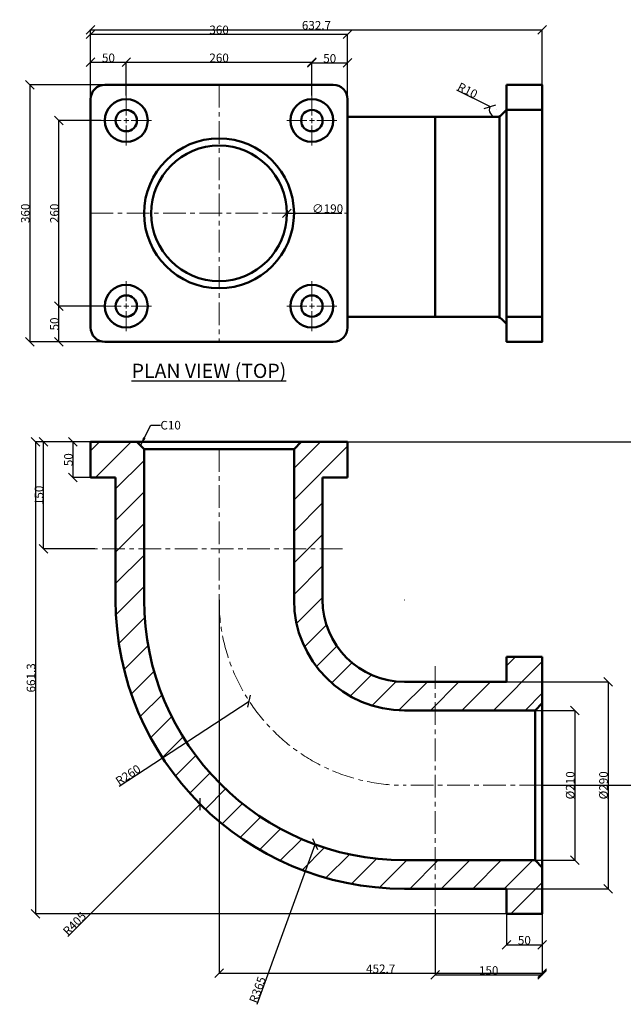
# Model space of a CAD drawing. Units: millimetres. Extents: x 509 to 2033, y 349 to 1731.
# Tile 1 of 2: x 509 to 1355, y 352 to 1731. Entities that reach past the tile are written whole.
import ezdxf

# ---------------------------------------------------------------- set-up
doc = ezdxf.new("R2010")
doc.units = ezdxf.units.MM
doc.header["$MEASUREMENT"] = 0
doc.linetypes.add('CENTER', pattern=[50.8, 31.75, -6.35, 6.35, -6.35])
for name, color, linetype, lineweight in [('M-CNTR', 1, 'CENTER', 18), ('M-DIMS', 2, 'Continuous', 25), ('M-HATC', 8, 'Continuous', 18), ('M-OUTL', 7, 'Continuous', 50), ('M-TEXT', 7, 'Continuous', 25)]:
    doc.layers.add(name, color=color, linetype=linetype, lineweight=lineweight)
doc.styles.get("Standard").update_dxf_attribs({"font": 'arial.ttf'})
doc.dimstyles.get("Standard").update_dxf_attribs({"dimtxt": 12, "dimasz": 12, "dimexe": 0.18, "dimexo": 0.0625, "dimgap": 0.09, "dimtad": 1, "dimdec": 0, "dimzin": 0, "dimdsep": 46, "dimtxsty": 'Standard', "dimblk": 'OBLIQUE', "dimcen": 0.09, "dimclre": 251, "dimadec": 0, "dimazin": 0, "dimtfac": 1, "dimtdec": 0, "dimtofl": 0, "dimtmove": 0, "dimatfit": 3, "dimfxl": 1, "dimtolj": 1, "dimtzin": 0, "dimarcsym": 0})

# ---------------------------------------------------------------- blocks, each defined once
blk = doc.blocks.new('*U2')
at = {"layer": 'M-CNTR', "color": 0, "transparency": 16777216}
for p, q in [((0, 7), (0, 35.12)), ((-35.12, 0), (-7, 0)), ((7, 0), (35.12, 0)), ((0, -35.12), (0, -7))]:
    blk.add_line(p, q, dxfattribs=at)
at = {"layer": 'M-CNTR', "color": 0, "linetype": 'Continuous', "transparency": 16777216}
for p, q in [((-3.5, 0), (3.5, 0)), ((0, -3.5), (0, 3.5))]:
    blk.add_line(p, q, dxfattribs=at)
blk = doc.blocks.new('*U3')
at = {"layer": 'M-CNTR', "color": 0, "transparency": 16777216}
for p, q in [((0, 7), (0, 35.12)), ((-35.12, 0), (-7, 0)), ((7, 0), (35.12, 0)), ((0, -35.12), (0, -7))]:
    blk.add_line(p, q, dxfattribs=at)
at = {"layer": 'M-CNTR', "color": 0, "linetype": 'Continuous', "transparency": 16777216}
for p, q in [((-3.5, 0), (3.5, 0)), ((0, -3.5), (0, 3.5))]:
    blk.add_line(p, q, dxfattribs=at)
blk = doc.blocks.new('*U4')
at = {"layer": 'M-CNTR', "color": 0, "transparency": 16777216}
for p, q in [((0, 7), (0, 35.12)), ((-35.12, 0), (-7, 0)), ((7, 0), (35.12, 0)), ((0, -35.12), (0, -7))]:
    blk.add_line(p, q, dxfattribs=at)
at = {"layer": 'M-CNTR', "color": 0, "linetype": 'Continuous', "transparency": 16777216}
for p, q in [((-3.5, 0), (3.5, 0)), ((0, -3.5), (0, 3.5))]:
    blk.add_line(p, q, dxfattribs=at)
blk = doc.blocks.new('*U5')
at = {"layer": 'M-CNTR', "color": 0, "transparency": 16777216}
for p, q in [((0, 7), (0, 35.12)), ((-35.12, 0), (-7, 0)), ((7, 0), (35.12, 0)), ((0, -35.12), (0, -7))]:
    blk.add_line(p, q, dxfattribs=at)
at = {"layer": 'M-CNTR', "color": 0, "linetype": 'Continuous', "transparency": 16777216}
for p, q in [((-3.5, 0), (3.5, 0)), ((0, -3.5), (0, 3.5))]:
    blk.add_line(p, q, dxfattribs=at)
blk = doc.blocks.new('_Oblique')
at = {"color": 0, "linetype": 'ByBlock', "lineweight": -2}
blk.add_line((-0.5, -0.5), (0.5, 0.5), dxfattribs=at)
blk = doc.blocks.new('*D10')
at = {"layer": 'Defpoints', "color": 0, "transparency": 16777216}
for p in [(563.7, 1590.1), (623.1, 1590.1), (623.1, 1330.1)]:
    blk.add_point(p, dxfattribs=at)
at = {"layer": 'M-DIMS', "color": 0, "lineweight": -2, "transparency": 16777216}
for p, q in [((623, 1590.1), (563.5, 1590.1)), ((563.7, 1330.1), (563.7, 1590.1)), ((623, 1330.1), (563.5, 1330.1))]:
    blk.add_line(p, q, dxfattribs=at)
at = {"layer": 'M-DIMS', "color": 0, "lineweight": -2, "transparency": 16777216, "xscale": 12, "yscale": 12, "zscale": 12}
for p, rotation in [((563.7, 1590.1), 90), ((563.7, 1330.1), 270)]:
    blk.add_blockref('_Oblique', p, dxfattribs=dict(at, rotation=rotation))
at = {"layer": 'M-DIMS', "color": 0, "transparency": 16777216, "insert": (557.5, 1460.1), "char_height": 12, "attachment_point": 5, "rotation": 90}
blk.add_mtext('\\A1;260', dxfattribs=at)
blk = doc.blocks.new('*D11')
at = {"layer": 'Defpoints', "color": 0, "transparency": 16777216}
for p in [(563.7, 1330.1), (628.2, 1330.1), (628.2, 1280.1)]:
    blk.add_point(p, dxfattribs=at)
at = {"layer": 'M-DIMS', "color": 0, "lineweight": -2, "transparency": 16777216}
for p, q in [((628.1, 1330.1), (563.5, 1330.1)), ((563.7, 1280.1), (563.7, 1330.1)), ((628.1, 1280.1), (563.5, 1280.1))]:
    blk.add_line(p, q, dxfattribs=at)
at = {"layer": 'M-DIMS', "color": 0, "lineweight": -2, "transparency": 16777216, "xscale": 12, "yscale": 12, "zscale": 12}
for p, rotation in [((563.7, 1330.1), 90), ((563.7, 1280.1), 270)]:
    blk.add_blockref('_Oblique', p, dxfattribs=dict(at, rotation=rotation))
at = {"layer": 'M-DIMS', "color": 0, "transparency": 16777216, "insert": (557.5, 1305.1), "char_height": 12, "attachment_point": 5, "rotation": 90}
blk.add_mtext('\\A1;50', dxfattribs=at)
blk = doc.blocks.new('*D12')
at = {"layer": 'Defpoints', "color": 0, "transparency": 16777216}
for p in [(628.2, 1640.1), (522.9, 1280.1), (639, 1280.1)]:
    blk.add_point(p, dxfattribs=at)
at = {"layer": 'M-DIMS', "color": 0, "lineweight": -2, "transparency": 16777216}
for p, q in [((628.1, 1640.1), (522.8, 1640.1)), ((522.9, 1640.1), (522.9, 1280.1)), ((639, 1280.1), (522.8, 1280.1))]:
    blk.add_line(p, q, dxfattribs=at)
at = {"layer": 'M-DIMS', "color": 0, "lineweight": -2, "transparency": 16777216, "xscale": 12, "yscale": 12, "zscale": 12}
for p, rotation in [((522.9, 1640.1), 90), ((522.9, 1280.1), 270)]:
    blk.add_blockref('_Oblique', p, dxfattribs=dict(at, rotation=rotation))
at = {"layer": 'M-DIMS', "color": 0, "transparency": 16777216, "insert": (516.7, 1460.1), "char_height": 12, "attachment_point": 5, "rotation": 90}
blk.add_mtext('\\A1;360', dxfattribs=at)
blk = doc.blocks.new('*D13')
at = {"layer": 'Defpoints', "color": 0, "transparency": 16777216}
for p in [(968.2, 1711), (608.2, 1620.1), (968.2, 1620.1)]:
    blk.add_point(p, dxfattribs=at)
at = {"layer": 'M-DIMS', "color": 0, "lineweight": -2, "transparency": 16777216}
for p, q in [((608.2, 1620.2), (608.2, 1711.2)), ((608.2, 1711), (968.2, 1711)), ((968.2, 1620.2), (968.2, 1711.2))]:
    blk.add_line(p, q, dxfattribs=at)
at = {"layer": 'M-DIMS', "color": 0, "lineweight": -2, "transparency": 16777216, "xscale": 12, "yscale": 12, "zscale": 12, "rotation": 180}
blk.add_blockref('_Oblique', (608.2, 1711), dxfattribs=at)
at = {"layer": 'M-DIMS', "color": 0, "lineweight": -2, "transparency": 16777216, "xscale": 12, "yscale": 12, "zscale": 12}
blk.add_blockref('_Oblique', (968.2, 1711), dxfattribs=at)
at = {"layer": 'M-DIMS', "color": 0, "transparency": 16777216, "insert": (788.2, 1717.2), "char_height": 12, "attachment_point": 5}
blk.add_mtext('\\A1;360', dxfattribs=at)
blk = doc.blocks.new('*D14')
at = {"layer": 'Defpoints', "color": 0, "transparency": 16777216}
for p in [(658.2, 1671.8), (608.2, 1620.1), (658.2, 1625.2)]:
    blk.add_point(p, dxfattribs=at)
at = {"layer": 'M-DIMS', "color": 0, "lineweight": -2, "transparency": 16777216}
for p, q in [((608.2, 1620.2), (608.2, 1672)), ((608.2, 1671.8), (658.2, 1671.8)), ((658.2, 1625.3), (658.2, 1672))]:
    blk.add_line(p, q, dxfattribs=at)
at = {"layer": 'M-DIMS', "color": 0, "lineweight": -2, "transparency": 16777216, "xscale": 12, "yscale": 12, "zscale": 12, "rotation": 180}
blk.add_blockref('_Oblique', (608.2, 1671.8), dxfattribs=at)
at = {"layer": 'M-DIMS', "color": 0, "lineweight": -2, "transparency": 16777216, "xscale": 12, "yscale": 12, "zscale": 12}
blk.add_blockref('_Oblique', (658.2, 1671.8), dxfattribs=at)
at = {"layer": 'M-DIMS', "color": 0, "transparency": 16777216, "insert": (633.2, 1678), "char_height": 12, "attachment_point": 5}
blk.add_mtext('\\A1;50', dxfattribs=at)
blk = doc.blocks.new('*D15')
at = {"layer": 'Defpoints', "color": 0, "transparency": 16777216}
for p in [(658.2, 1671.8), (918.2, 1671.8), (918.2, 1625.2)]:
    blk.add_point(p, dxfattribs=at)
at = {"layer": 'M-DIMS', "color": 0, "lineweight": -2, "transparency": 16777216}
for p, q in [((658.2, 1671.9), (658.2, 1672)), ((658.2, 1671.8), (918.2, 1671.8)), ((918.2, 1625.3), (918.2, 1672))]:
    blk.add_line(p, q, dxfattribs=at)
at = {"layer": 'M-DIMS', "color": 0, "lineweight": -2, "transparency": 16777216, "xscale": 12, "yscale": 12, "zscale": 12, "rotation": 180}
blk.add_blockref('_Oblique', (658.2, 1671.8), dxfattribs=at)
at = {"layer": 'M-DIMS', "color": 0, "lineweight": -2, "transparency": 16777216, "xscale": 12, "yscale": 12, "zscale": 12}
blk.add_blockref('_Oblique', (918.2, 1671.8), dxfattribs=at)
at = {"layer": 'M-DIMS', "color": 0, "transparency": 16777216, "insert": (788.2, 1678), "char_height": 12, "attachment_point": 5}
blk.add_mtext('\\A1;260', dxfattribs=at)
blk = doc.blocks.new('*D16')
at = {"layer": 'Defpoints', "color": 0, "transparency": 16777216}
for p in [(968.2, 1671), (918.2, 1625.2), (968.2, 1620.1)]:
    blk.add_point(p, dxfattribs=at)
at = {"layer": 'M-DIMS', "color": 0, "lineweight": -2, "transparency": 16777216}
for p, q in [((918.2, 1625.3), (918.2, 1671.1)), ((918.2, 1671), (968.2, 1671)), ((968.2, 1620.2), (968.2, 1671.1))]:
    blk.add_line(p, q, dxfattribs=at)
at = {"layer": 'M-DIMS', "color": 0, "lineweight": -2, "transparency": 16777216, "xscale": 12, "yscale": 12, "zscale": 12, "rotation": 180}
blk.add_blockref('_Oblique', (918.2, 1671), dxfattribs=at)
at = {"layer": 'M-DIMS', "color": 0, "lineweight": -2, "transparency": 16777216, "xscale": 12, "yscale": 12, "zscale": 12}
blk.add_blockref('_Oblique', (968.2, 1671), dxfattribs=at)
at = {"layer": 'M-DIMS', "color": 0, "transparency": 16777216, "insert": (943.2, 1677.2), "char_height": 12, "attachment_point": 5}
blk.add_mtext('\\A1;50', dxfattribs=at)
blk = doc.blocks.new('*D17')
at = {"layer": 'Defpoints', "color": 0, "transparency": 16777216}
for p in [(1167.8, 1609.6), (1176.8, 1605.1)]:
    blk.add_point(p, dxfattribs=at)
at = {"layer": 'M-DIMS', "color": 0, "lineweight": -2, "transparency": 16777216}
for p, q in [((1120.6, 1633.2), (1167.8, 1609.6)), ((1176.7, 1605.1), (1176.9, 1605.1)), ((1176.8, 1605), (1176.8, 1605.2))]:
    blk.add_line(p, q, dxfattribs=at)
blk.add_arc((1176.8, 1605.1), 10, 152.4068, 269.6419, dxfattribs=at)
at = {"layer": 'M-DIMS', "color": 0, "lineweight": -2, "transparency": 16777216, "xscale": 12, "yscale": 12, "zscale": 12, "rotation": 333.4380769186279}
blk.add_blockref('_Oblique', (1167.8, 1609.6), dxfattribs=at)
at = {"layer": 'M-DIMS', "color": 0, "transparency": 16777216, "insert": (1136.3, 1632.3), "char_height": 12, "attachment_point": 5, "rotation": 333.4381}
blk.add_mtext('\\A1;R10', dxfattribs=at)
blk = doc.blocks.new('*D18')
at = {"layer": 'Defpoints', "color": 0, "transparency": 16777216}
for p in [(542.1, 1139.9), (608.2, 1139.9), (614.3, 989.9)]:
    blk.add_point(p, dxfattribs=at)
at = {"layer": 'M-DIMS', "color": 0, "lineweight": -2, "transparency": 16777216}
for p, q in [((608.1, 1139.9), (541.9, 1139.9)), ((542.1, 989.9), (542.1, 1139.9)), ((614.2, 989.9), (541.9, 989.9))]:
    blk.add_line(p, q, dxfattribs=at)
at = {"layer": 'M-DIMS', "color": 0, "lineweight": -2, "transparency": 16777216, "xscale": 12, "yscale": 12, "zscale": 12}
for p, rotation in [((542.1, 1139.9), 90), ((542.1, 989.9), 270)]:
    blk.add_blockref('_Oblique', p, dxfattribs=dict(at, rotation=rotation))
at = {"layer": 'M-DIMS', "color": 0, "transparency": 16777216, "insert": (535.9, 1064.9), "char_height": 12, "attachment_point": 5, "rotation": 90}
blk.add_mtext('\\A1;150', dxfattribs=at)
blk = doc.blocks.new('*D19')
at = {"layer": 'Defpoints', "color": 0, "transparency": 16777216}
for p in [(608.2, 1139.9), (583.3, 1089.9), (608.2, 1089.9)]:
    blk.add_point(p, dxfattribs=at)
at = {"layer": 'M-DIMS', "color": 0, "lineweight": -2, "transparency": 16777216}
for p, q in [((608.1, 1139.9), (583.1, 1139.9)), ((583.3, 1139.9), (583.3, 1089.9)), ((608.1, 1089.9), (583.1, 1089.9))]:
    blk.add_line(p, q, dxfattribs=at)
at = {"layer": 'M-DIMS', "color": 0, "lineweight": -2, "transparency": 16777216, "xscale": 12, "yscale": 12, "zscale": 12}
for p, rotation in [((583.3, 1139.9), 90), ((583.3, 1089.9), 270)]:
    blk.add_blockref('_Oblique', p, dxfattribs=dict(at, rotation=rotation))
at = {"layer": 'M-DIMS', "color": 0, "transparency": 16777216, "insert": (577.1, 1114.9), "char_height": 12, "attachment_point": 5, "rotation": 90}
blk.add_mtext('\\A1;50', dxfattribs=at)
blk = doc.blocks.new('*D20')
at = {"layer": 'Defpoints', "color": 0, "transparency": 16777216}
for p in [(1048.2, 918.6), (830.4, 776.5)]:
    blk.add_point(p, dxfattribs=at)
at = {"layer": 'M-DIMS', "color": 0, "lineweight": -2, "transparency": 16777216}
for p, q in [((1048.1, 918.6), (1048.3, 918.6)), ((1048.2, 918.5), (1048.2, 918.7)), ((648.1, 657.6), (830.4, 776.5))]:
    blk.add_line(p, q, dxfattribs=at)
at = {"layer": 'M-DIMS', "color": 0, "lineweight": -2, "transparency": 16777216, "xscale": 12, "yscale": 12, "zscale": 12, "rotation": 33.11996082454108}
blk.add_blockref('_Oblique', (830.4, 776.5), dxfattribs=at)
at = {"layer": 'M-DIMS', "color": 0, "transparency": 16777216, "insert": (660.7, 673.2), "char_height": 12, "attachment_point": 5, "rotation": 33.12}
blk.add_mtext('\\A1;R260', dxfattribs=at)
blk = doc.blocks.new('*D21')
at = {"layer": 'Defpoints', "color": 0, "transparency": 16777216}
for p in [(1190.9, 478.6), (1240.9, 478.6), (1240.9, 435.2)]:
    blk.add_point(p, dxfattribs=at)
at = {"layer": 'M-DIMS', "color": 0, "lineweight": -2, "transparency": 16777216}
for p, q in [((1190.9, 478.5), (1190.9, 435)), ((1240.9, 478.5), (1240.9, 435)), ((1190.9, 435.2), (1240.9, 435.2))]:
    blk.add_line(p, q, dxfattribs=at)
at = {"layer": 'M-DIMS', "color": 0, "lineweight": -2, "transparency": 16777216, "xscale": 12, "yscale": 12, "zscale": 12, "rotation": 180}
blk.add_blockref('_Oblique', (1190.9, 435.2), dxfattribs=at)
at = {"layer": 'M-DIMS', "color": 0, "lineweight": -2, "transparency": 16777216, "xscale": 12, "yscale": 12, "zscale": 12}
blk.add_blockref('_Oblique', (1240.9, 435.2), dxfattribs=at)
at = {"layer": 'M-DIMS', "color": 0, "transparency": 16777216, "insert": (1215.9, 441.4), "char_height": 12, "attachment_point": 5}
blk.add_mtext('\\A1;50', dxfattribs=at)
blk = doc.blocks.new('*D22')
at = {"layer": 'Defpoints', "color": 0, "transparency": 16777216}
for p in [(1090.9, 484.9), (1240.9, 478.6), (1240.9, 392.9)]:
    blk.add_point(p, dxfattribs=at)
at = {"layer": 'M-DIMS', "color": 0, "lineweight": -2, "transparency": 16777216}
for p, q in [((1090.9, 484.9), (1090.9, 392.7)), ((1240.9, 478.5), (1240.9, 392.7)), ((1090.9, 392.9), (1240.9, 392.9))]:
    blk.add_line(p, q, dxfattribs=at)
at = {"layer": 'M-DIMS', "color": 0, "lineweight": -2, "transparency": 16777216, "xscale": 12, "yscale": 12, "zscale": 12, "rotation": 180}
blk.add_blockref('_Oblique', (1090.9, 392.9), dxfattribs=at)
at = {"layer": 'M-DIMS', "color": 0, "lineweight": -2, "transparency": 16777216, "xscale": 12, "yscale": 12, "zscale": 12}
blk.add_blockref('_Oblique', (1240.9, 392.9), dxfattribs=at)
at = {"layer": 'M-DIMS', "color": 0, "transparency": 16777216, "insert": (1165.9, 399.1), "char_height": 12, "attachment_point": 5}
blk.add_mtext('\\A1;150', dxfattribs=at)
blk = doc.blocks.new('*D23')
at = {"layer": 'Defpoints', "color": 0, "transparency": 16777216}
for p in [(1230.9, 763.6), (1230.9, 553.6), (1286.6, 553.6)]:
    blk.add_point(p, dxfattribs=at)
at = {"layer": 'M-DIMS', "color": 0, "lineweight": -2, "transparency": 16777216}
for p, q in [((1231, 763.6), (1286.8, 763.6)), ((1286.6, 763.6), (1286.6, 553.6)), ((1231, 553.6), (1286.8, 553.6))]:
    blk.add_line(p, q, dxfattribs=at)
at = {"layer": 'M-DIMS', "color": 0, "lineweight": -2, "transparency": 16777216, "xscale": 12, "yscale": 12, "zscale": 12}
for p, rotation in [((1286.6, 763.6), 90), ((1286.6, 553.6), 270)]:
    blk.add_blockref('_Oblique', p, dxfattribs=dict(at, rotation=rotation))
at = {"layer": 'M-DIMS', "color": 0, "transparency": 16777216, "insert": (1280.1, 658.6), "char_height": 12, "attachment_point": 5, "rotation": 90}
blk.add_mtext('\\A1;%%C210', dxfattribs=at)
blk = doc.blocks.new('*D24')
at = {"layer": 'Defpoints', "color": 0, "transparency": 16777216}
for p in [(1190.9, 803.6), (1190.9, 513.6), (1333.3, 513.6)]:
    blk.add_point(p, dxfattribs=at)
at = {"layer": 'M-DIMS', "color": 0, "lineweight": -2, "transparency": 16777216}
for p, q in [((1191, 803.6), (1333.5, 803.6)), ((1333.3, 803.6), (1333.3, 513.6)), ((1191, 513.6), (1333.5, 513.6))]:
    blk.add_line(p, q, dxfattribs=at)
at = {"layer": 'M-DIMS', "color": 0, "lineweight": -2, "transparency": 16777216, "xscale": 12, "yscale": 12, "zscale": 12}
for p, rotation in [((1333.3, 803.6), 90), ((1333.3, 513.6), 270)]:
    blk.add_blockref('_Oblique', p, dxfattribs=dict(at, rotation=rotation))
at = {"layer": 'M-DIMS', "color": 0, "transparency": 16777216, "insert": (1326.7, 658.6), "char_height": 12, "attachment_point": 5, "rotation": 90}
blk.add_mtext('\\A1;%%C290', dxfattribs=at)
blk = doc.blocks.new('BOLT-HOLE-CBORE')
for radius in [30, 15]:
    blk.add_circle((30, 30), radius)
blk = doc.blocks.new('*D35')
at = {"layer": 'Defpoints', "color": 0, "transparency": 16777216}
for p in [(968.2, 1139.9), (1240.9, 658.6), (1981, 658.6)]:
    blk.add_point(p, dxfattribs=at)
at = {"layer": 'M-DIMS', "color": 251, "lineweight": -2, "transparency": 16777216}
for p, q in [((968.2, 1139.9), (1981.1, 1139.9)), ((1241, 658.6), (1981.1, 658.6))]:
    blk.add_line(p, q, dxfattribs=at)
at = {"layer": 'M-DIMS', "color": 0, "lineweight": -2, "transparency": 16777216}
blk.add_line((1981, 1139.9), (1981, 658.6), dxfattribs=at)
at = {"layer": 'M-DIMS', "color": 0, "lineweight": -2, "transparency": 16777216, "xscale": 12, "yscale": 12, "zscale": 12}
for p, rotation in [((1981, 1139.9), 90), ((1981, 658.6), 270)]:
    blk.add_blockref('_Oblique', p, dxfattribs=dict(at, rotation=rotation))
at = {"layer": 'M-DIMS', "color": 0, "transparency": 16777216, "insert": (1974.7, 899.2), "char_height": 12, "attachment_point": 5, "rotation": 90}
blk.add_mtext('\\A1;481.3', dxfattribs=at)
blk = doc.blocks.new('*D36')
at = {"layer": 'Defpoints', "color": 0, "transparency": 16777216}
for p in [(788.2, 918.6), (1240.9, 478.6), (1240.9, 395.3)]:
    blk.add_point(p, dxfattribs=at)
at = {"layer": 'M-DIMS', "color": 251, "lineweight": -2, "transparency": 16777216}
for p, q in [((788.2, 918.5), (788.2, 395.1)), ((1240.9, 478.5), (1240.9, 395.1))]:
    blk.add_line(p, q, dxfattribs=at)
at = {"layer": 'M-DIMS', "color": 0, "lineweight": -2, "transparency": 16777216}
blk.add_line((788.2, 395.3), (1240.9, 395.3), dxfattribs=at)
at = {"layer": 'M-DIMS', "color": 0, "lineweight": -2, "transparency": 16777216, "xscale": 12, "yscale": 12, "zscale": 12, "rotation": 180}
blk.add_blockref('_Oblique', (788.2, 395.3), dxfattribs=at)
at = {"layer": 'M-DIMS', "color": 0, "lineweight": -2, "transparency": 16777216, "xscale": 12, "yscale": 12, "zscale": 12}
blk.add_blockref('_Oblique', (1240.9, 395.3), dxfattribs=at)
at = {"layer": 'M-DIMS', "color": 0, "transparency": 16777216, "insert": (1014.6, 401.5), "char_height": 12, "attachment_point": 5}
blk.add_mtext('\\A1;452.7', dxfattribs=at)
blk = doc.blocks.new('*D37')
at = {"layer": 'Defpoints', "color": 0, "transparency": 16777216}
for p in [(608.2, 1139.9), (530.9, 478.6), (1240.9, 478.6)]:
    blk.add_point(p, dxfattribs=at)
at = {"layer": 'M-DIMS', "color": 251, "lineweight": -2, "transparency": 16777216}
for p, q in [((608.1, 1139.9), (530.8, 1139.9)), ((1240.9, 478.6), (530.8, 478.6))]:
    blk.add_line(p, q, dxfattribs=at)
at = {"layer": 'M-DIMS', "color": 0, "lineweight": -2, "transparency": 16777216}
blk.add_line((530.9, 1139.9), (530.9, 478.6), dxfattribs=at)
at = {"layer": 'M-DIMS', "color": 0, "lineweight": -2, "transparency": 16777216, "xscale": 12, "yscale": 12, "zscale": 12}
for p, rotation in [((530.9, 1139.9), 90), ((530.9, 478.6), 270)]:
    blk.add_blockref('_Oblique', p, dxfattribs=dict(at, rotation=rotation))
at = {"layer": 'M-DIMS', "color": 0, "transparency": 16777216, "insert": (524.7, 809.2), "char_height": 12, "attachment_point": 5, "rotation": 90}
blk.add_mtext('\\A1;661.3', dxfattribs=at)
blk = doc.blocks.new('*D38')
at = {"layer": 'Defpoints', "color": 0, "transparency": 16777216}
for p in [(1240.9, 1717.4), (1240.9, 1640.1), (608.2, 1620.1)]:
    blk.add_point(p, dxfattribs=at)
at = {"layer": 'M-DIMS', "color": 251, "lineweight": -2, "transparency": 16777216}
for p, q in [((608.2, 1620.2), (608.2, 1717.6)), ((1240.9, 1640.2), (1240.9, 1717.6))]:
    blk.add_line(p, q, dxfattribs=at)
at = {"layer": 'M-DIMS', "color": 0, "lineweight": -2, "transparency": 16777216}
blk.add_line((608.2, 1717.4), (1240.9, 1717.4), dxfattribs=at)
at = {"layer": 'M-DIMS', "color": 0, "lineweight": -2, "transparency": 16777216, "xscale": 12, "yscale": 12, "zscale": 12, "rotation": 180}
blk.add_blockref('_Oblique', (608.2, 1717.4), dxfattribs=at)
at = {"layer": 'M-DIMS', "color": 0, "lineweight": -2, "transparency": 16777216, "xscale": 12, "yscale": 12, "zscale": 12}
blk.add_blockref('_Oblique', (1240.9, 1717.4), dxfattribs=at)
at = {"layer": 'M-DIMS', "color": 0, "transparency": 16777216, "insert": (924.6, 1723.6), "char_height": 12, "attachment_point": 5}
blk.add_mtext('\\A1;632.7', dxfattribs=at)
blk = doc.blocks.new('*D39')
at = {"layer": 'Defpoints', "color": 0, "transparency": 16777216}
for p in [(1048.2, 918.6), (761.8, 632.2)]:
    blk.add_point(p, dxfattribs=at)
at = {"layer": 'M-DIMS', "color": 251, "lineweight": -2, "transparency": 16777216}
for p, q in [((1048.1, 918.6), (1048.3, 918.6)), ((1048.2, 918.5), (1048.2, 918.7))]:
    blk.add_line(p, q, dxfattribs=at)
at = {"layer": 'M-DIMS', "color": 0, "lineweight": -2, "transparency": 16777216}
blk.add_line((576.4, 446.9), (761.8, 632.2), dxfattribs=at)
at = {"layer": 'M-DIMS', "color": 0, "lineweight": -2, "transparency": 16777216, "xscale": 12, "yscale": 12, "zscale": 12, "rotation": 44.99999749912137}
blk.add_blockref('_Oblique', (761.8, 632.2), dxfattribs=at)
at = {"layer": 'M-DIMS', "color": 0, "transparency": 16777216, "insert": (585.6, 464.8), "char_height": 12, "attachment_point": 5, "rotation": 45}
blk.add_mtext('\\A1;R405', dxfattribs=at)
blk = doc.blocks.new('*D40')
at = {"layer": 'Defpoints', "color": 0, "transparency": 16777216}
for p in [(1048.2, 918.6), (923, 575.7)]:
    blk.add_point(p, dxfattribs=at)
at = {"layer": 'M-DIMS', "color": 251, "lineweight": -2, "transparency": 16777216}
for p, q in [((1048.1, 918.6), (1048.3, 918.6)), ((1048.2, 918.5), (1048.2, 918.7))]:
    blk.add_line(p, q, dxfattribs=at)
at = {"layer": 'M-DIMS', "color": 0, "lineweight": -2, "transparency": 16777216}
blk.add_line((841.4, 352), (923, 575.7), dxfattribs=at)
at = {"layer": 'M-DIMS', "color": 0, "lineweight": -2, "transparency": 16777216, "xscale": 12, "yscale": 12, "zscale": 12, "rotation": 69.95038313699236}
blk.add_blockref('_Oblique', (923, 575.7), dxfattribs=at)
at = {"layer": 'M-DIMS', "color": 0, "transparency": 16777216, "insert": (842.1, 372.1), "char_height": 12, "attachment_point": 5, "rotation": 69.9504}
blk.add_mtext('\\A1;R365', dxfattribs=at)
blk = doc.blocks.new('*D41')
at = {"layer": 'Defpoints', "color": 0, "transparency": 16777216}
for p in [(693.2, 1460.1), (883.2, 1460.1)]:
    blk.add_point(p, dxfattribs=at)
at = {"layer": 'M-DIMS', "color": 251, "lineweight": -2, "transparency": 16777216}
for p, q in [((788.1, 1460.1), (788.3, 1460.1)), ((788.2, 1460), (788.2, 1460.2))]:
    blk.add_line(p, q, dxfattribs=at)
at = {"layer": 'M-DIMS', "color": 0, "lineweight": -2, "transparency": 16777216}
blk.add_line((960, 1460.1), (883.2, 1460.1), dxfattribs=at)
at = {"layer": 'M-DIMS', "color": 0, "lineweight": -2, "transparency": 16777216, "xscale": 12, "yscale": 12, "zscale": 12, "rotation": 180.0001025292896}
blk.add_blockref('_Oblique', (883.2, 1460.1), dxfattribs=at)
at = {"layer": 'M-DIMS', "color": 0, "transparency": 16777216, "insert": (940.2, 1466.7), "char_height": 12, "attachment_point": 5, "rotation": 0.0001}
blk.add_mtext('\\A1;∅190', dxfattribs=at)

msp = doc.modelspace()

# ---------------------------------------------------------------- hatches: boundary and pattern name
at = {"layer": 'M-HATC'}
h = msp.add_hatch(dxfattribs=at)
h.set_pattern_fill('ANSI31', color=256, scale=250)
h.set_pattern_definition([(45, (92.202, 1053.204), (-22.0971, 22.0971), [])])
h.paths.add_polyline_path([(683.18, 1129.86), (673.18, 1139.86), (608.18, 1139.86), (608.18, 1089.86), (643.18, 1089.86), (643.18, 989.86), (683.18, 989.86)])
h.paths.add_polyline_path([(933.18, 1089.86), (968.18, 1089.86), (968.18, 1139.86), (903.18, 1139.86), (893.18, 1129.86), (893.18, 989.86), (933.18, 989.86)])
h.paths.add_polyline_path([(933.18, 918.61), (933.18, 989.86), (893.18, 989.86), (893.18, 918.61, 0.4142136), (1048.18, 763.61), (1230.92, 763.61), (1240.92, 773.61), (1240.92, 838.61), (1190.92, 838.61), (1190.92, 803.61), (1048.18, 803.61, -0.4142136)])
h.paths.add_polyline_path([(1240.92, 543.61), (1230.92, 553.61), (1048.18, 553.61, -0.4142136), (683.18, 918.61), (683.18, 989.86), (643.18, 989.86), (643.18, 918.61, 0.4142136), (1048.18, 513.61), (1190.92, 513.61), (1190.92, 478.61), (1240.92, 478.61)])

# ---------------------------------------------------------------- linework, layer by layer
at = {"layer": 'M-CNTR'}
for p, q in [((788.18, 1640.13), (788.18, 1280.13)), ((608.18, 1460.13), (968.18, 1460.13)), ((788.18, 1129.86), (788.18, 918.61)), ((960.98, 989.86), (614.3, 989.86)), ((1090.92, 825.75), (1090.92, 484.93)), ((1240.92, 658.61), (1048.18, 658.61))]:
    msp.add_line(p, q, dxfattribs=at)
msp.add_arc((1048.18, 918.61), 260, 180, 270, dxfattribs=at)
at = {"layer": 'M-OUTL'}
for p, q in [((1190.92, 1605.13), (1183.85, 1598.06)), ((1190.92, 1605.13), (1240.92, 1605.13)), ((1176.78, 1595.13), (968.18, 1595.13)), ((1090.92, 1315.13), (1090.92, 1595.13)), ((1180.92, 1314.23), (1180.92, 1596.03)), ((1176.78, 1315.13), (968.18, 1315.13)), ((1183.85, 1312.2), (1190.92, 1305.13)), ((1240.92, 1315.13), (1190.92, 1315.13)), ((608.18, 1139.86), (968.18, 1139.86)), ((608.18, 1139.86), (608.18, 1089.86)), ((673.18, 1139.86), (683.18, 1129.86)), ((893.18, 1129.86), (903.18, 1139.86)), ((968.18, 1139.86), (968.18, 1089.86)), ((683.18, 918.61), (683.18, 1129.86)), ((683.18, 1129.86), (893.18, 1129.86)), ((893.18, 918.61), (893.18, 1129.86)), ((608.18, 1089.86), (643.18, 1089.86)), ((643.18, 1089.86), (643.18, 918.61)), ((933.18, 1089.86), (968.18, 1089.86)), ((933.18, 1089.86), (933.18, 918.61)), ((1190.92, 838.61), (1190.92, 803.61)), ((1240.92, 838.61), (1190.92, 838.61)), ((1240.92, 838.61), (1240.92, 478.61)), ((1190.92, 803.61), (1048.18, 803.61)), ((1240.92, 773.61), (1230.92, 763.61)), ((1048.18, 763.61), (1230.92, 763.61)), ((1230.92, 763.61), (1230.92, 553.61)), ((1048.18, 553.61), (1230.92, 553.61)), ((1240.92, 543.61), (1230.92, 553.61)), ((1190.92, 513.61), (1048.18, 513.61)), ((1190.92, 513.61), (1190.92, 478.61)), ((1240.92, 478.61), (1190.92, 478.61))]:
    msp.add_line(p, q, dxfattribs=at)
msp.add_lwpolyline([(628.18, 1640.13), (948.18, 1640.13, -0.4142136), (968.18, 1620.13), (968.18, 1300.13, -0.4142136), (948.18, 1280.13), (628.18, 1280.13, -0.4142136), (608.18, 1300.13), (608.18, 1620.13, -0.4142136)], format="xyb", close=True, dxfattribs=at)
msp.add_lwpolyline([(1190.92, 1640.13), (1240.92, 1640.13), (1240.92, 1280.13), (1190.92, 1280.13)], close=True, dxfattribs=at)
for centre, radius in [((658.18, 1590.13), 30), ((788.18, 1460.13), 105), ((788.18, 1460.13), 95)]:
    msp.add_circle(centre, radius, dxfattribs=at)
for centre, radius, start, end in [((1176.78, 1605.13), 10, 270, 315), ((1176.78, 1305.13), 10, 45, 90), ((1048.18, 918.61), 405, 180, 270), ((1048.18, 918.61), 365, 180, 270), ((1048.18, 918.61), 155, 180, 270), ((1048.18, 918.61), 115, 180, 270)]:
    msp.add_arc(centre, radius, start, end, dxfattribs=at)

# ---------------------------------------------------------------- block references
at = {"layer": 'M-CNTR'}
for name, p in [('*U4', (658.18, 1590.13)), ('*U5', (918.18, 1590.13)), ('*U3', (658.18, 1330.13)), ('*U2', (918.18, 1330.13))]:
    msp.add_blockref(name, p, dxfattribs=at)
at = {"layer": 'M-OUTL'}
for p in [(628.18, 1560.13), (888.18, 1560.13), (628.18, 1300.13), (888.18, 1300.13)]:
    msp.add_blockref('BOLT-HOLE-CBORE', p, dxfattribs=at)

# ---------------------------------------------------------------- texts
at = {"layer": 'M-TEXT'}
for s, insert, char_height, attachment_point in [('\\A1;{\\LPLAN VIEW (TOP)}', (774.02, 1239.43), 20, 5), ('C10', (705.99, 1169.23), 12, 1)]:
    msp.add_mtext(s, dxfattribs=dict(at, insert=insert, char_height=char_height, attachment_point=attachment_point))

# ---------------------------------------------------------------- dimensions: what is measured, and where the dimension line sits
at = {"layer": 'M-DIMS'}
for base, p1, p2, override, picture, middle in [((1240.92, 1717.38), (608.18, 1620.13), (1240.92, 1640.13), {"dimdec": 1, "dimlfac": 1, "dimrnd": 0, "dimzin": 0, "dimdsep": 46, "dimlunit": 2}, '*D38', (924.55, 1723.6)), ((968.18, 1711.03), (608.18, 1620.13), (968.18, 1620.13), {"dimclrd": 0, "dimclre": 0, "dimclrt": 0}, '*D13', (788.18, 1717.25)), ((658.18, 1671.79), (608.18, 1620.13), (658.18, 1625.25), {"dimclrd": 0, "dimclre": 0, "dimclrt": 0}, '*D14', (633.18, 1678.01)), ((918.18, 1671.79), (658.18, 1671.79), (918.18, 1625.25), {"dimclrd": 0, "dimclre": 0, "dimclrt": 0}, '*D15', (788.18, 1678.01)), ((968.18, 1670.96), (918.18, 1625.25), (968.18, 1620.13), {"dimclrd": 0, "dimclre": 0, "dimclrt": 0}, '*D16', (943.18, 1677.18)), ((1240.92, 395.26), (788.18, 918.61), (1240.92, 478.61), {"dimdec": 1, "dimlfac": 1, "dimrnd": 0, "dimzin": 0, "dimdsep": 46, "dimlunit": 2}, '*D36', (1014.55, 401.47)), ((1240.92, 392.89), (1090.92, 484.93), (1240.92, 478.61), {"dimclrd": 0, "dimclre": 0, "dimclrt": 0}, '*D22', (1165.92, 399.11)), ((1240.92, 435.23), (1190.92, 478.61), (1240.92, 478.61), {"dimclrd": 0, "dimclre": 0, "dimclrt": 0}, '*D21', (1215.92, 441.44))]:
    dim = msp.add_linear_dim(base=base, p1=p1, p2=p2, dimstyle='Standard', override=override, dxfattribs=at)
    dim.commit()
    dim.dimension.update_dxf_attribs({"geometry": picture, "text_midpoint": middle})
for base, p1, p2, override, picture, middle in [((522.95, 1280.13), (628.18, 1640.13), (639.01, 1280.13), {"dimclrd": 0, "dimclre": 0, "dimclrt": 0}, '*D12', (516.73, 1460.13)), ((563.68, 1590.13), (623.06, 1330.13), (623.06, 1590.13), {"dimclrd": 0, "dimclre": 0, "dimclrt": 0}, '*D10', (557.47, 1460.13)), ((563.68, 1330.13), (628.18, 1280.13), (628.18, 1330.13), {"dimclrd": 0, "dimclre": 0, "dimclrt": 0}, '*D11', (557.47, 1305.13)), ((530.9301, 478.6051), (608.1801, 1139.8615), (1240.9212, 478.6051), {"dimdec": 1, "dimlfac": 1, "dimrnd": 0, "dimzin": 0, "dimdsep": 46, "dimlunit": 2}, '*D37', (524.7092, 809.2333)), ((542.08, 1139.86), (614.3, 989.86), (608.18, 1139.86), {"dimclrd": 0, "dimclre": 0, "dimclrt": 0}, '*D18', (535.86, 1064.86)), ((583.28, 1089.86), (608.18, 1139.86), (608.18, 1089.86), {"dimclrd": 0, "dimclre": 0, "dimclrt": 0}, '*D19', (577.07, 1114.86)), ((1980.9517, 658.6051), (968.1801, 1139.8615), (1240.9212, 658.6051), {"dimdec": 1, "dimlfac": 1, "dimrnd": 0, "dimzin": 0, "dimdsep": 46, "dimlunit": 2}, '*D35', (1974.7307, 899.2333))]:
    dim = msp.add_linear_dim(base=base, p1=p1, p2=p2, angle=90, dimstyle='Standard', override=override, dxfattribs=at)
    dim.commit()
    dim.dimension.update_dxf_attribs({"geometry": picture, "text_midpoint": middle})
dim = msp.add_radius_dim(center=(1176.78, 1605.13), mpoint=(1167.84, 1609.6), dimstyle='Standard', override={"dimclrd": 0, "dimclre": 0, "dimclrt": 0}, dxfattribs=at)
dim.commit()
dim.dimension.update_dxf_attribs({"geometry": '*D17', "text_midpoint": (1136.26, 1632.33)})
dim = msp.add_diameter_dim_2p(p1=(693.18, 1460.13), p2=(883.18, 1460.13), dimstyle='Standard', override={"dimdec": 0, "dimlfac": 1, "dimrnd": 0, "dimzin": 0, "dimdsep": 46, "dimlunit": 2}, dxfattribs=at)
dim.commit()
dim.dimension.update_dxf_attribs({"geometry": '*D41', "text_midpoint": (940.18, 1460.13), "dimtype": 163})
for mpoint, override, picture, middle in [((761.8, 632.23), {"dimdec": 0, "dimlfac": 1, "dimrnd": 0, "dimzin": 0, "dimdsep": 46, "dimlunit": 2}, '*D39', (589.97, 460.4)), ((830.42, 776.54), {"dimclrd": 0, "dimclre": 0, "dimclrt": 0}, '*D20', (664.11, 668.04)), ((923.05, 575.73), {"dimdec": 0, "dimlfac": 1, "dimrnd": 0, "dimzin": 0, "dimdsep": 46, "dimlunit": 2}, '*D40', (847.97, 370))]:
    dim = msp.add_radius_dim(center=(1048.18, 918.61), mpoint=mpoint, dimstyle='Standard', override=override, dxfattribs=at)
    dim.commit()
    dim.dimension.update_dxf_attribs({"geometry": picture, "text_midpoint": middle, "dimtype": 164})
for base, p1, p2, picture, middle in [((1333.27, 513.61), (1190.92, 803.61), (1190.92, 513.61), '*D24', (1326.72, 658.61)), ((1286.63, 553.61), (1230.92, 763.61), (1230.92, 553.61), '*D23', (1280.08, 658.61))]:
    dim = msp.add_linear_dim(base=base, p1=p1, p2=p2, angle=90, text='%%C<>', dimstyle='Standard', override={"dimclrd": 0, "dimclre": 0, "dimclrt": 0}, dxfattribs=at)
    dim.commit()
    dim.dimension.update_dxf_attribs({"geometry": picture, "text_midpoint": middle})

# ---------------------------------------------------------------- leaders
at = {"layer": 'M-DIMS', "annotation_type": 0, "has_hookline": 1, "hookline_direction": 1, "text_width": 29.12}
msp.add_leader([(678.18, 1134.86), (692.4, 1163.23), (705.9, 1163.23)], dimstyle='Standard', override={"dimgap": 0.09, "dimtad": 0}, dxfattribs=at)

doc.saveas('drawing.dxf')
